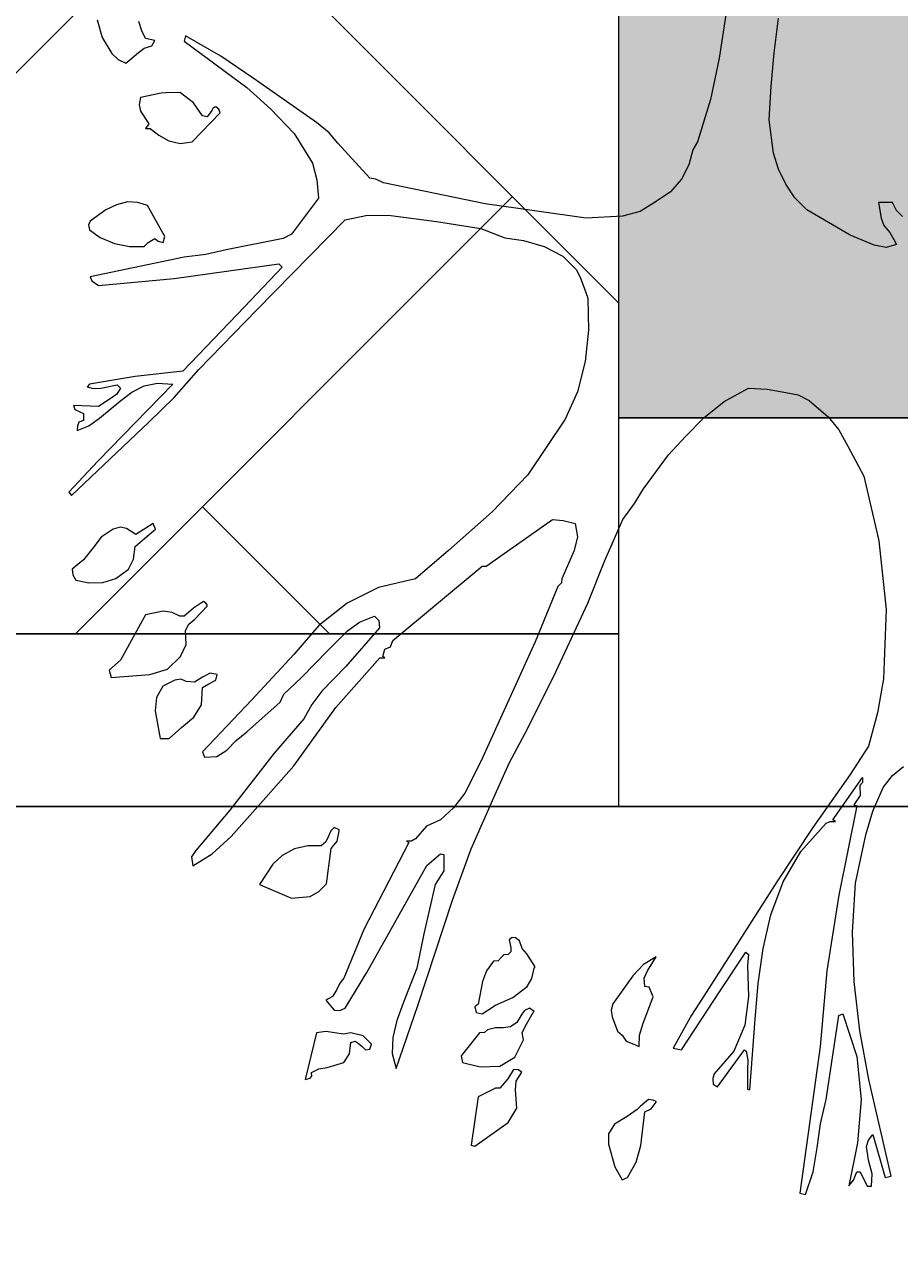
# Model space of a CAD drawing. Units: inches. Extents: x 84 to 1044, y -280 to 906.
# Tile 3 of 105: x 441 to 462, y -132 to -104. Entities that reach past the tile are written whole.
import ezdxf

# ---------------------------------------------------------------- set-up
doc = ezdxf.new("R2010")
doc.units = ezdxf.units.IN
for name, color, linetype, lineweight in [('A-ANNO-DIMS', 2, 'Continuous', 18), ('C-PROP', 7, 'Continuous', 25), ('L-HRDS', 32, 'Continuous', 18), ('L-PLNT', 114, 'Continuous', 15)]:
    doc.layers.add(name, color=color, linetype=linetype, lineweight=lineweight)
doc.layers.add('L-PLNT-PATT', color=9, linetype='Continuous', lineweight=9, true_color=0xafd9aa)
doc.layers.add('L-PRKG-PATT', color=35, linetype='Continuous', lineweight=9, true_color=0x947764)
doc.styles.get("Standard").update_dxf_attribs({"font": 'arial.ttf'})
doc.dimstyles.get("Standard").update_dxf_attribs({"dimtxt": 0.18, "dimasz": 0.18, "dimexe": 0.18, "dimexo": 0.0625, "dimgap": 0.09, "dimtad": 0, "dimtih": 1, "dimtoh": 1, "dimdec": 4, "dimzin": 0, "dimdsep": 46, "dimtxsty": 'Standard', "dimcen": 0.09, "dimadec": 0, "dimazin": 0, "dimtfac": 1, "dimtdec": 4, "dimtofl": 0, "dimtmove": 0, "dimatfit": 3, "dimfxl": 1, "dimtolj": 1, "dimtzin": 0, "dimarcsym": 0})

# ---------------------------------------------------------------- blocks, each defined once
blk = doc.blocks.new('A$C37E508DF')
for p, q in [((0.7911, 1.1436), (0.8027, 1.0677)), ((0.7512, 1.0728), (0.7469, 1.1054)), ((1.3455, 1.0934), (1.3485, 1.102)), ((1.3875, 1.1037), (1.3828, 1.087)), ((1.2713, 1.0694), (1.3044, 1.0887)), ((1.3044, 1.0887), (1.3057, 1.0835)), ((1.3421, 1.0861), (1.3455, 1.0934)), ((1.3057, 1.0835), (1.2469, 1.0402)), ((1.3335, 1.0844), (1.3421, 1.0861)), ((1.3361, 1.0793), (1.3335, 1.0844)), ((1.3434, 1.0771), (1.3361, 1.0793)), ((1.349, 1.0728), (1.3434, 1.0771)), ((1.3828, 1.087), (1.3738, 1.072)), ((0.7538, 1.0415), (0.7512, 1.0728)), ((0.8027, 1.0677), (0.8108, 1.0287)), ((1.2409, 1.0488), (1.2713, 1.0694)), ((1.3605, 1.063), (1.349, 1.0728)), ((1.3678, 1.0664), (1.3605, 1.063)), ((1.3738, 1.072), (1.3678, 1.0664)), ((1.1813, 1.0072), (1.2409, 1.0488)), ((0.7559, 1.0098), (0.7538, 1.0415)), ((1.2469, 1.0402), (1.2246, 1.0201)), ((1.2971, 1.0257), (1.3091, 1.0351)), ((1.3091, 1.0351), (1.3185, 1.0355)), ((1.3185, 1.0355), (1.3275, 1.0347)), ((1.3275, 1.0347), (1.3468, 1.0308)), ((0.8108, 1.0287), (0.8233, 0.9892)), ((1.2246, 1.0201), (1.2023, 0.9969)), ((1.2718, 1.0162), (1.2731, 1.0197)), ((1.2731, 1.0197), (1.2761, 1.0218)), ((1.2761, 1.0218), (1.2786, 1.0209)), ((1.2786, 1.0209), (1.2799, 1.0184)), ((1.2885, 1.0136), (1.2971, 1.0257)), ((1.3468, 1.0308), (1.3481, 1.0239)), ((1.3481, 1.0239), (1.3468, 1.018)), ((0.7516, 0.9785), (0.7559, 1.0098)), ((1.2984, 0.9892), (1.2718, 1.0162)), ((1.2799, 1.0184), (1.2842, 1.0124)), ((1.2842, 1.0124), (1.2885, 1.0136)), ((1.3468, 1.018), (1.3391, 1.0059)), ((1.1612, 0.9879), (1.1693, 0.9974)), ((1.1693, 0.9974), (1.1813, 1.0072)), ((1.2023, 0.9969), (1.1852, 0.9691)), ((1.3378, 1.0016), (1.3297, 0.9952)), ((1.3421, 1.0016), (1.3378, 1.0016)), ((1.3391, 1.0059), (1.3421, 1.0016)), ((0.8233, 0.9892), (0.8275, 0.9815)), ((1.1311, 0.9549), (1.1612, 0.9879)), ((1.3095, 0.9875), (1.2984, 0.9892)), ((1.3202, 0.9901), (1.3095, 0.9875)), ((1.3297, 0.9952), (1.3202, 0.9901)), ((0.7469, 0.9635), (0.7516, 0.9785)), ((0.8275, 0.9815), (0.8314, 0.9673)), ((0.7401, 0.9493), (0.7469, 0.9635)), ((0.8314, 0.9673), (0.8383, 0.954)), ((1.1852, 0.9691), (1.1809, 0.9532)), ((0.8383, 0.954), (0.8486, 0.942)), ((1.1183, 0.9506), (1.1256, 0.954)), ((1.1256, 0.954), (1.1311, 0.9549)), ((1.1809, 0.9532), (1.1796, 0.936)), ((0.7315, 0.9365), (0.7401, 0.9493)), ((0.8486, 0.942), (0.8619, 0.933)), ((1.0227, 0.9309), (1.1183, 0.9506)), ((0.6359, 0.9245), (0.6397, 0.9322)), ((0.6397, 0.9322), (0.653, 0.9322)), ((0.653, 0.9322), (0.6505, 0.9172)), ((0.7203, 0.9253), (0.7315, 0.9365)), ((0.8619, 0.933), (0.8769, 0.9236)), ((0.9279, 0.9172), (1.0227, 0.9309)), ((1.1796, 0.936), (1.2049, 0.9022)), ((1.3241, 0.9), (1.3404, 0.9292)), ((1.3404, 0.9292), (1.3494, 0.9322)), ((1.3494, 0.9322), (1.3592, 0.9326)), ((1.3592, 0.9326), (1.3695, 0.93)), ((1.3695, 0.93), (1.3794, 0.9253)), ((0.6303, 0.9189), (0.6359, 0.9245)), ((0.6505, 0.9172), (0.6479, 0.9103)), ((0.6796, 0.9013), (0.7203, 0.9253)), ((0.8769, 0.9236), (0.8936, 0.9193)), ((0.8936, 0.9193), (0.9279, 0.9172)), ((1.1114, 0.9198), (1.0685, 0.9142)), ((1.1333, 0.9202), (1.1114, 0.9198)), ((1.1543, 0.9159), (1.1333, 0.9202)), ((1.3794, 0.9253), (1.394, 0.9146)), ((0.6479, 0.9103), (0.6423, 0.9039)), ((1.0269, 0.9077), (1.0042, 0.8987)), ((1.0685, 0.9142), (1.0269, 0.9077)), ((1.2371, 0.8314), (1.1543, 0.9159)), ((1.3948, 0.9065), (1.3846, 0.8992)), ((1.394, 0.9146), (1.3957, 0.9112)), ((1.3957, 0.9112), (1.3948, 0.9065)), ((0.6384, 0.8974), (0.6359, 0.8927)), ((0.6423, 0.9039), (0.6384, 0.8974)), ((0.6569, 0.8919), (0.6796, 0.9013)), ((0.9866, 0.8962), (0.9673, 0.8906)), ((1.0042, 0.8987), (0.9866, 0.8962)), ((1.2049, 0.9022), (1.2126, 0.8983)), ((1.2126, 0.8983), (1.2662, 0.8876)), ((1.3254, 0.8944), (1.3241, 0.9)), ((1.3301, 0.8957), (1.3254, 0.8944)), ((1.3335, 0.8983), (1.3301, 0.8957)), ((1.3395, 0.8944), (1.3335, 0.8983)), ((1.3434, 0.8906), (1.3395, 0.8944)), ((1.3713, 0.8936), (1.3571, 0.8906)), ((1.3846, 0.8992), (1.3713, 0.8936)), ((0.6359, 0.8927), (0.6457, 0.8897)), ((0.6457, 0.8897), (0.6569, 0.8919)), ((0.9673, 0.8906), (0.9498, 0.8816)), ((1.2662, 0.8876), (1.2855, 0.8833)), ((1.2855, 0.8833), (1.3057, 0.8807)), ((1.3571, 0.8906), (1.3434, 0.8906)), ((0.9498, 0.8816), (0.9369, 0.8687)), ((1.2169, 0.8743), (1.2135, 0.8713)), ((1.2135, 0.8713), (1.2491, 0.834)), ((1.3151, 0.8606), (1.2169, 0.8743)), ((1.3057, 0.8807), (1.394, 0.8623)), ((0.933, 0.861), (0.9296, 0.852)), ((0.9369, 0.8687), (0.933, 0.861)), ((1.3863, 0.8541), (1.3151, 0.8606)), ((1.394, 0.8623), (1.3927, 0.8584)), ((0.9296, 0.852), (0.9262, 0.8421)), ((1.3927, 0.8584), (1.3863, 0.8541)), ((0.9262, 0.8421), (0.9257, 0.8121)), ((1.2919, 0.7752), (1.2371, 0.8314)), ((1.2491, 0.834), (1.3069, 0.7735)), ((0.9257, 0.8121), (0.9287, 0.7825)), ((0.9287, 0.7825), (0.936, 0.7542)), ((1.3151, 0.7487), (1.2919, 0.7752)), ((1.3069, 0.7735), (1.352, 0.7684)), ((1.352, 0.7684), (1.3948, 0.7615)), ((0.7577, 0.7568), (0.7401, 0.7534)), ((0.7752, 0.7577), (0.7577, 0.7568)), ((0.798, 0.7452), (0.7752, 0.7577)), ((1.3309, 0.7624), (1.3164, 0.7615)), ((1.3164, 0.7615), (1.3871, 0.6891)), ((1.3434, 0.7598), (1.3309, 0.7624)), ((1.355, 0.7538), (1.3434, 0.7598)), ((1.3687, 0.7607), (1.3657, 0.7577)), ((1.3657, 0.7577), (1.3691, 0.7521)), ((1.3841, 0.7577), (1.3687, 0.7607)), ((1.3914, 0.7572), (1.3841, 0.7577)), ((1.397, 0.759), (1.3914, 0.7572)), ((1.3948, 0.7615), (1.397, 0.759)), ((0.7182, 0.7461), (0.7002, 0.7307)), ((0.7285, 0.7512), (0.7182, 0.7461)), ((0.7401, 0.7534), (0.7285, 0.7512)), ((0.8173, 0.7298), (0.798, 0.7452)), ((0.936, 0.7542), (0.9476, 0.7285)), ((1.3391, 0.7255), (1.3151, 0.7487)), ((1.3653, 0.7461), (1.355, 0.7538)), ((1.3854, 0.7294), (1.3653, 0.7461)), ((1.3691, 0.7521), (1.3743, 0.7482)), ((1.3743, 0.7482), (1.3863, 0.7405)), ((1.3863, 0.7405), (1.4099, 0.7414)), ((1.4086, 0.7375), (1.4004, 0.7337)), ((1.4004, 0.7337), (1.4004, 0.7272)), ((1.4099, 0.7414), (1.4086, 0.7375)), ((0.7002, 0.7307), (0.6903, 0.7186)), ((0.8344, 0.7122), (0.8173, 0.7298)), ((0.9476, 0.7285), (0.9828, 0.6762)), ((1.4116, 0.6569), (1.3391, 0.7255)), ((1.3953, 0.7221), (1.3854, 0.7294)), ((1.4064, 0.7178), (1.3953, 0.7221)), ((1.4004, 0.7272), (1.4047, 0.7255)), ((1.4047, 0.7255), (1.406, 0.7221)), ((1.406, 0.7221), (1.4064, 0.7178)), ((0.6903, 0.7186), (0.6818, 0.7032)), ((0.8503, 0.6951), (0.8344, 0.7122)), ((0.6818, 0.7032), (0.6667, 0.6749)), ((0.8739, 0.6629), (0.8503, 0.6951)), ((1.3871, 0.6891), (1.4141, 0.6599)), ((0.9828, 0.6762), (1.0162, 0.6415)), ((0.6667, 0.6749), (0.6526, 0.614)), ((0.8824, 0.6492), (0.8739, 0.6629)), ((1.4141, 0.6599), (1.4116, 0.6569)), ((0.8932, 0.6342), (0.8824, 0.6492)), ((0.9103, 0.5956), (0.8932, 0.6342)), ((0.9382, 0.6303), (0.936, 0.6179)), ((0.9493, 0.6333), (0.9382, 0.6303)), ((0.9596, 0.6342), (0.9493, 0.6333)), ((1.0218, 0.5904), (0.9596, 0.6342)), ((1.0162, 0.6415), (1.0574, 0.605)), ((1.3327, 0.6252), (1.3348, 0.6303)), ((1.3348, 0.6303), (1.3511, 0.62)), ((1.343, 0.6162), (1.3327, 0.6252)), ((1.3511, 0.62), (1.3601, 0.6256)), ((1.3601, 0.6256), (1.3661, 0.6269)), ((1.3661, 0.6269), (1.3725, 0.6252)), ((1.3725, 0.6252), (1.3837, 0.6175)), ((0.6526, 0.614), (0.6457, 0.5497)), ((0.936, 0.6179), (0.939, 0.605)), ((1.352, 0.6089), (1.343, 0.6162)), ((1.3533, 0.5969), (1.352, 0.6089)), ((1.3837, 0.6175), (1.3918, 0.6072)), ((0.939, 0.605), (0.9506, 0.5784)), ((1.0574, 0.605), (1.0883, 0.5784)), ((1.358, 0.5874), (1.3533, 0.5969)), ((1.3918, 0.6072), (1.4004, 0.5964)), ((1.4004, 0.5964), (1.4111, 0.5874)), ((0.9262, 0.5557), (0.9103, 0.5956)), ((1.0256, 0.5904), (1.0218, 0.5904)), ((1.1097, 0.5205), (1.0256, 0.5904)), ((1.37, 0.5789), (1.358, 0.5874)), ((1.4111, 0.5874), (1.4103, 0.5823)), ((0.9506, 0.5784), (0.951, 0.5746)), ((0.951, 0.5746), (0.9545, 0.5711)), ((1.0883, 0.5784), (1.123, 0.5703)), ((1.3824, 0.575), (1.37, 0.5789)), ((1.3953, 0.5746), (1.3824, 0.575)), ((1.4077, 0.5771), (1.3953, 0.5746)), ((1.4103, 0.5823), (1.4077, 0.5771)), ((0.9545, 0.5711), (0.9759, 0.5193)), ((1.123, 0.5703), (1.1526, 0.5557)), ((0.9583, 0.4871), (0.9262, 0.5557)), ((1.1526, 0.5557), (1.1792, 0.5347)), ((1.2842, 0.554), (1.2855, 0.5557)), ((1.2842, 0.5527), (1.2842, 0.554)), ((1.2958, 0.5407), (1.2842, 0.5527)), ((1.2855, 0.5557), (1.2876, 0.557)), ((1.2876, 0.557), (1.2971, 0.551)), ((1.2971, 0.551), (1.3057, 0.5433)), ((0.6457, 0.5497), (0.6483, 0.4845)), ((1.1226, 0.5394), (1.1221, 0.5325)), ((1.1268, 0.5433), (1.1226, 0.5394)), ((1.141, 0.5377), (1.1268, 0.5433)), ((1.3014, 0.536), (1.2958, 0.5407)), ((1.3057, 0.5433), (1.3099, 0.5433)), ((1.3099, 0.5433), (1.3172, 0.5467)), ((1.3172, 0.5467), (1.3254, 0.548)), ((1.3254, 0.548), (1.3421, 0.5446)), ((1.3421, 0.5446), (1.3657, 0.5021)), ((1.1221, 0.5325), (1.1539, 0.4961)), ((1.1521, 0.5296), (1.141, 0.5377)), ((1.1706, 0.5111), (1.1521, 0.5296)), ((1.1792, 0.5347), (1.2027, 0.5072)), ((1.3044, 0.53), (1.3014, 0.536)), ((1.3039, 0.5167), (1.3044, 0.53)), ((0.9759, 0.5193), (1.0269, 0.4069)), ((1.1118, 0.5145), (1.1097, 0.5205)), ((1.3091, 0.5055), (1.3039, 0.5167)), ((1.117, 0.5124), (1.1118, 0.5145)), ((1.1191, 0.5055), (1.117, 0.5124)), ((1.117, 0.5042), (1.1191, 0.5055)), ((1.1217, 0.5042), (1.117, 0.5042)), ((1.1633, 0.4575), (1.1217, 0.5042)), ((1.1955, 0.4858), (1.1706, 0.5111)), ((1.2027, 0.5072), (1.2426, 0.4644)), ((1.3215, 0.4935), (1.3091, 0.5055)), ((1.1539, 0.4961), (1.1762, 0.4729)), ((1.3382, 0.4884), (1.3215, 0.4935)), ((1.3657, 0.5021), (1.3764, 0.4927)), ((1.3764, 0.4927), (1.3743, 0.4858)), ((0.6483, 0.4845), (0.6539, 0.4524)), ((0.9853, 0.4335), (0.9583, 0.4871)), ((1.207, 0.4747), (1.1955, 0.4858)), ((1.2748, 0.4884), (1.2812, 0.4897)), ((1.2761, 0.4832), (1.2748, 0.4884)), ((1.2825, 0.4798), (1.2761, 0.4832)), ((1.2812, 0.4897), (1.2885, 0.4862)), ((1.2885, 0.4862), (1.2962, 0.4815)), ((1.2962, 0.4815), (1.3039, 0.482)), ((1.3039, 0.482), (1.3087, 0.4841)), ((1.3087, 0.4841), (1.3147, 0.4832)), ((1.3147, 0.4832), (1.3258, 0.4777)), ((1.3743, 0.4858), (1.3382, 0.4884)), ((1.1762, 0.4729), (1.1856, 0.4605)), ((1.2122, 0.47), (1.207, 0.4747)), ((1.2156, 0.4627), (1.2122, 0.47)), ((1.2885, 0.4764), (1.2825, 0.4798)), ((1.2894, 0.4601), (1.2885, 0.4764)), ((1.3258, 0.4777), (1.3318, 0.4669)), ((1.1856, 0.4605), (1.1933, 0.4468)), ((1.2469, 0.4348), (1.2156, 0.4627)), ((1.2426, 0.4644), (1.2885, 0.4159)), ((1.2967, 0.4485), (1.2894, 0.4601)), ((1.3318, 0.4669), (1.3331, 0.4545)), ((0.6539, 0.4524), (0.6625, 0.4211)), ((1.2027, 0.4026), (1.1633, 0.4575)), ((1.1933, 0.4468), (1.2212, 0.4146)), ((1.3082, 0.4386), (1.2967, 0.4485)), ((1.3331, 0.4545), (1.3284, 0.4284)), ((1.3198, 0.4284), (1.3082, 0.4386)), ((1.0003, 0.4052), (0.9853, 0.4335)), ((1.2568, 0.4266), (1.2469, 0.4348)), ((1.2658, 0.4176), (1.2568, 0.4266)), ((1.3284, 0.4284), (1.3198, 0.4284)), ((0.6625, 0.4211), (0.6796, 0.3945)), ((1.2212, 0.4146), (1.2628, 0.361)), ((1.2752, 0.4116), (1.2658, 0.4176)), ((1.2885, 0.4159), (1.2868, 0.4108)), ((0.6397, 0.3936), (0.6295, 0.4022)), ((1.0145, 0.373), (1.0003, 0.4052)), ((1.0269, 0.4069), (1.0419, 0.3769)), ((1.2289, 0.373), (1.2027, 0.4026)), ((1.2868, 0.4108), (1.2752, 0.4116)), ((0.6487, 0.3825), (0.6397, 0.3936)), ((0.6959, 0.352), (0.668, 0.3919)), ((0.668, 0.3919), (0.668, 0.3872)), ((0.6796, 0.3945), (0.7148, 0.3447)), ((0.6582, 0.3602), (0.6487, 0.3825)), ((0.668, 0.3872), (0.6706, 0.3842)), ((0.6706, 0.3842), (0.6702, 0.3748)), ((0.6702, 0.3748), (0.6762, 0.3662)), ((1.0359, 0.3246), (1.0145, 0.373)), ((1.0419, 0.3769), (1.0527, 0.3632)), ((1.2615, 0.3362), (1.2289, 0.373)), ((0.665, 0.3379), (0.6582, 0.3602)), ((0.6762, 0.3662), (0.6732, 0.3653)), ((0.6732, 0.3653), (0.6903, 0.2813)), ((1.0527, 0.3632), (1.0647, 0.352)), ((1.2628, 0.361), (1.2949, 0.3233)), ((0.6933, 0.3503), (0.6959, 0.352)), ((0.6985, 0.3503), (0.6933, 0.3503)), ((0.7023, 0.349), (0.6985, 0.3503)), ((0.7259, 0.3224), (0.7023, 0.349)), ((0.7148, 0.3447), (0.7487, 0.2937)), ((1.0647, 0.352), (1.078, 0.346)), ((1.078, 0.346), (1.0883, 0.334)), ((1.1599, 0.3426), (1.1646, 0.3447)), ((1.1646, 0.3447), (1.168, 0.3417)), ((0.6745, 0.2924), (0.665, 0.3379)), ((1.0883, 0.334), (1.0921, 0.3319)), ((1.1599, 0.3413), (1.1599, 0.3426)), ((1.162, 0.3319), (1.1599, 0.3413)), ((1.168, 0.3417), (1.1702, 0.3366)), ((1.1702, 0.3366), (1.1727, 0.3314)), ((1.2795, 0.3199), (1.2615, 0.3362)), ((0.7427, 0.2937), (0.7259, 0.3224)), ((1.0535, 0.2766), (1.0359, 0.3246)), ((1.0921, 0.3319), (1.0968, 0.3319)), ((1.0968, 0.3319), (1.0947, 0.3306)), ((1.0947, 0.3306), (1.1367, 0.2491)), ((1.1676, 0.325), (1.162, 0.3319)), ((1.1719, 0.292), (1.1676, 0.325)), ((1.1727, 0.3314), (1.177, 0.3276)), ((1.177, 0.3276), (1.1895, 0.3276)), ((1.1895, 0.3276), (1.2019, 0.3246)), ((1.2019, 0.3246), (1.2135, 0.3186)), ((1.2949, 0.3233), (1.2988, 0.3173)), ((1.0647, 0.3199), (1.0617, 0.3194)), ((1.0617, 0.3194), (1.0617, 0.304)), ((1.0711, 0.3147), (1.0647, 0.3199)), ((1.0775, 0.3092), (1.0711, 0.3147)), ((1.2135, 0.3186), (1.2225, 0.3104)), ((1.2225, 0.3104), (1.2349, 0.2911)), ((1.2975, 0.3087), (1.2795, 0.3199)), ((1.2988, 0.3173), (1.2975, 0.3087)), ((1.0617, 0.304), (1.0698, 0.2911)), ((1.1341, 0.2084), (1.0775, 0.3092)), ((0.6775, 0.2465), (0.6745, 0.2924)), ((0.7542, 0.2628), (0.7427, 0.2937)), ((0.7487, 0.2937), (0.8151, 0.1899)), ((1.0698, 0.2911), (1.0805, 0.2448)), ((1.1792, 0.2847), (1.1719, 0.292)), ((1.2349, 0.2911), (1.2049, 0.2783)), ((0.6903, 0.2813), (0.7015, 0.2101)), ((1.0861, 0.1775), (1.0535, 0.2766)), ((1.1873, 0.28), (1.1792, 0.2847)), ((1.2049, 0.2783), (1.1873, 0.28)), ((0.7615, 0.2311), (0.7542, 0.2628)), ((0.6758, 0.2002), (0.6775, 0.2465)), ((0.9905, 0.2384), (0.9943, 0.241)), ((0.9943, 0.241), (0.9973, 0.2414)), ((0.9973, 0.2414), (1.0003, 0.2393)), ((1.0805, 0.2448), (1.087, 0.2127)), ((1.1367, 0.2491), (1.1556, 0.2032)), ((0.7662, 0.1981), (0.7615, 0.2311)), ((0.9836, 0.226), (0.9879, 0.2311)), ((0.9879, 0.2311), (0.9905, 0.2384)), ((1.0003, 0.2393), (0.9986, 0.232)), ((0.9986, 0.232), (0.9986, 0.2281)), ((0.7778, 0.2277), (0.7752, 0.2255)), ((0.7752, 0.2255), (0.7761, 0.2152)), ((0.8018, 0.1912), (0.7778, 0.2277)), ((0.8619, 0.2234), (0.8739, 0.2161)), ((0.87, 0.2101), (0.8619, 0.2234)), ((0.9759, 0.214), (0.9836, 0.226)), ((0.9986, 0.2281), (1.0012, 0.2255)), ((1.0012, 0.2255), (1.0051, 0.2251)), ((1.0051, 0.2251), (1.0076, 0.2225)), ((1.0076, 0.2225), (1.0106, 0.2195)), ((1.0106, 0.2195), (1.0149, 0.2191)), ((1.0149, 0.2191), (1.0214, 0.2101)), ((0.7015, 0.2101), (0.7079, 0.1389)), ((0.7761, 0.2152), (0.7752, 0.1861)), ((0.8734, 0.2032), (0.87, 0.2101)), ((0.8739, 0.2161), (0.8841, 0.2054)), ((0.9768, 0.2127), (0.9759, 0.214)), ((0.9789, 0.2028), (0.9768, 0.2127)), ((1.0214, 0.2101), (1.0252, 0.2002)), ((1.087, 0.2127), (1.0998, 0.1797)), ((1.1543, 0.1749), (1.1341, 0.2084)), ((0.6706, 0.1539), (0.6758, 0.2002)), ((0.7688, 0.1646), (0.7662, 0.1981)), ((0.8687, 0.1947), (0.8726, 0.1955)), ((0.8726, 0.1955), (0.8734, 0.2032)), ((0.8841, 0.2054), (0.9026, 0.1792)), ((0.9832, 0.1955), (0.9789, 0.2028)), ((0.9969, 0.1852), (0.9832, 0.1955)), ((1.0252, 0.2002), (1.0295, 0.1788)), ((1.1556, 0.2032), (1.1594, 0.1985)), ((1.1594, 0.1985), (1.1624, 0.1921)), ((0.7752, 0.1861), (0.7787, 0.1591)), ((0.8383, 0.1359), (0.8018, 0.1912)), ((0.8151, 0.1899), (0.8288, 0.1685)), ((0.8649, 0.1857), (0.8687, 0.1947)), ((0.8743, 0.1608), (0.8649, 0.1857)), ((1.0132, 0.1779), (0.9969, 0.1852)), ((1.1624, 0.1921), (1.1663, 0.1861)), ((1.1663, 0.1861), (1.1727, 0.1827)), ((0.9026, 0.1792), (0.9043, 0.1732)), ((0.9043, 0.1732), (0.9035, 0.1668)), ((0.9768, 0.1719), (0.9811, 0.1749)), ((0.9776, 0.1711), (0.9768, 0.1719)), ((0.9811, 0.1749), (0.9858, 0.1728)), ((0.9858, 0.1728), (0.9884, 0.1694)), ((1.0256, 0.1698), (1.0132, 0.1779)), ((1.0295, 0.1788), (1.0325, 0.1762)), ((1.0325, 0.1762), (1.0312, 0.1711)), ((1.1063, 0.1183), (1.0861, 0.1775)), ((1.0998, 0.1797), (1.1058, 0.1634)), ((1.1594, 0.1728), (1.1543, 0.1749)), ((1.1646, 0.1732), (1.1594, 0.1728)), ((1.1727, 0.1827), (1.1646, 0.1732)), ((0.6865, 0.1698), (0.6732, 0.1295)), ((0.6903, 0.1681), (0.6865, 0.1698)), ((0.7023, 0.0892), (0.6903, 0.1681)), ((0.774, 0.0982), (0.7688, 0.1646)), ((0.8288, 0.1685), (0.846, 0.1376)), ((0.8777, 0.1496), (0.8743, 0.1608)), ((0.9035, 0.1668), (0.8983, 0.1535)), ((0.9853, 0.1578), (0.9776, 0.1711)), ((0.9884, 0.1694), (0.9931, 0.1616)), ((0.9931, 0.1616), (0.9991, 0.1574)), ((1.0312, 0.1711), (1.0256, 0.1698)), ((1.1058, 0.1634), (1.1097, 0.1475)), ((0.662, 0.108), (0.6706, 0.1539)), ((0.7787, 0.1591), (0.789, 0.1346)), ((0.8781, 0.1389), (0.8777, 0.1496)), ((0.894, 0.1496), (0.8902, 0.1441)), ((0.8983, 0.1535), (0.894, 0.1496)), ((0.9879, 0.1518), (0.9853, 0.1578)), ((0.9866, 0.1453), (0.9879, 0.1518)), ((0.9991, 0.1574), (1.0059, 0.1565)), ((1.0059, 0.1565), (1.0132, 0.1565)), ((1.0132, 0.1565), (1.0205, 0.1548)), ((1.0205, 0.1548), (1.0235, 0.1522)), ((1.0235, 0.1522), (1.0282, 0.1518)), ((1.0282, 0.1518), (1.0454, 0.1303)), ((1.1298, 0.1411), (1.1376, 0.1492)), ((1.1376, 0.1492), (1.1491, 0.1518)), ((1.1491, 0.1518), (1.1564, 0.1505)), ((1.1564, 0.1505), (1.1642, 0.1518)), ((1.1642, 0.1518), (1.1727, 0.1531)), ((1.1727, 0.1531), (1.1813, 0.1518)), ((1.1813, 0.1518), (1.192, 0.108)), ((0.7079, 0.1389), (0.7268, 0.0013)), ((0.846, 0.1376), (0.8383, 0.1359)), ((0.8846, 0.1419), (0.8781, 0.1389)), ((0.8902, 0.1441), (0.8846, 0.1419)), ((0.9948, 0.1291), (0.9866, 0.1453)), ((1.1097, 0.1475), (1.1101, 0.1325)), ((1.1311, 0.1364), (1.1298, 0.1411)), ((1.1384, 0.1389), (1.1354, 0.1359)), ((1.1423, 0.1423), (1.1384, 0.1389)), ((1.1449, 0.1441), (1.1423, 0.1423)), ((1.1491, 0.1428), (1.1449, 0.1441)), ((1.1504, 0.132), (1.1491, 0.1428)), ((0.6732, 0.1295), (0.6693, 0.0892)), ((0.7774, 0.1346), (0.7757, 0.1261)), ((0.7757, 0.1261), (0.7761, 0.117)), ((0.7791, 0.1359), (0.7774, 0.1346)), ((0.8044, 0.1012), (0.7791, 0.1359)), ((0.789, 0.1346), (0.8074, 0.1132)), ((1.0089, 0.1205), (0.9948, 0.1291)), ((1.0454, 0.1303), (1.0441, 0.1239)), ((1.1101, 0.1325), (1.1063, 0.1183)), ((1.1354, 0.1359), (1.1311, 0.1364)), ((1.1556, 0.1239), (1.1504, 0.132)), ((0.7761, 0.117), (0.7761, 0.099)), ((0.9884, 0.1149), (0.9918, 0.117)), ((0.9935, 0.1063), (0.9884, 0.1149)), ((0.9918, 0.117), (0.9961, 0.1175)), ((0.9961, 0.1175), (1.0016, 0.1085)), ((1.0274, 0.12), (1.0089, 0.1205)), ((1.0441, 0.1239), (1.0274, 0.12)), ((1.1714, 0.1192), (1.1556, 0.1239)), ((1.1792, 0.1179), (1.1714, 0.1192)), ((1.186, 0.1145), (1.1792, 0.1179)), ((0.641, 0.0172), (0.662, 0.108)), ((0.8083, 0.1037), (0.8044, 0.1012)), ((0.8074, 0.1132), (0.8087, 0.1089)), ((0.8087, 0.1089), (0.8083, 0.1037)), ((0.9943, 0.0982), (0.9935, 0.1063)), ((1.0016, 0.1085), (1.0089, 0.0999)), ((1.1856, 0.111), (1.186, 0.1145)), ((1.1873, 0.1093), (1.1856, 0.111)), ((1.192, 0.108), (1.1873, 0.1093)), ((0.7761, 0.099), (0.774, 0.0982)), ((0.9931, 0.081), (0.9943, 0.0982)), ((1.0089, 0.0999), (1.0132, 0.0999)), ((1.0132, 0.0999), (1.0295, 0.0917)), ((1.0295, 0.0917), (1.0359, 0.0463)), ((0.6693, 0.0892), (0.6728, 0.0484)), ((0.7075, 0.0665), (0.7023, 0.0892)), ((0.8619, 0.0875), (0.8649, 0.0887)), ((0.8619, 0.0866), (0.8619, 0.0875)), ((0.8666, 0.0806), (0.8619, 0.0866)), ((0.8649, 0.0887), (0.8691, 0.0892)), ((0.8726, 0.0776), (0.8666, 0.0806)), ((0.8691, 0.0892), (0.8769, 0.0827)), ((0.8769, 0.0827), (0.8799, 0.0797)), ((1.0012, 0.0677), (0.9931, 0.081)), ((0.8764, 0.0459), (0.8726, 0.0776)), ((0.8799, 0.0797), (0.8893, 0.0733)), ((0.8893, 0.0733), (0.9013, 0.066)), ((0.7105, 0.0437), (0.7075, 0.0665)), ((0.9013, 0.066), (0.9069, 0.057)), ((1.0325, 0.0454), (1.0012, 0.0677)), ((0.6582, 0.0562), (0.6466, 0.0159)), ((0.6625, 0.051), (0.6582, 0.0562)), ((0.6642, 0.045), (0.6625, 0.051)), ((0.6728, 0.0484), (0.6809, 0.0082)), ((0.8807, 0.0304), (0.8764, 0.0459)), ((0.9069, 0.0471), (0.9009, 0.0261)), ((0.9069, 0.057), (0.9069, 0.0471)), ((1.0359, 0.0463), (1.0325, 0.0454)), ((0.6625, 0.0321), (0.6642, 0.045)), ((0.7144, 0.0214), (0.7105, 0.0437)), ((0.659, 0.0193), (0.6625, 0.0321)), ((0.8889, 0.0159), (0.8807, 0.0304)), ((0.9009, 0.0261), (0.894, 0.0137)), ((0.6466, 0.0159), (0.641, 0.0172)), ((0.6595, 0.0077), (0.659, 0.0193)), ((0.6702, 0.0214), (0.6637, 0.0077)), ((0.6732, 0.0214), (0.6702, 0.0214)), ((0.6766, 0.0133), (0.6732, 0.0214)), ((0.6809, 0.0082), (0.6766, 0.0133)), ((0.7216, 0), (0.7144, 0.0214)), ((0.894, 0.0137), (0.8889, 0.0159)), ((0.6637, 0.0077), (0.6595, 0.0077)), ((0.7268, 0.0013), (0.7216, 0))]:
    blk.add_line(p, q)
blk = doc.blocks.new('*D60')
at = {"layer": 'A-ANNO-DIMS', "color": 0, "lineweight": -2, "transparency": 16777216}
for p, q in [((134.179, -121.942), (134.179, -180.64)), ((992.074, -121.942), (992.074, -180.64)), ((134.359, -180.46), (562.733, -180.46)), ((991.894, -180.46), (563.521, -180.46))]:
    blk.add_line(p, q, dxfattribs=at)
at = {"layer": 'A-ANNO-DIMS', "color": 0, "transparency": 16777216}
for points in [[(134.359, -180.43), (134.359, -180.49), (134.179, -180.46)], [(991.894, -180.43), (991.894, -180.49), (992.074, -180.46)]]:
    blk.add_solid(points, dxfattribs=at)
at = {"layer": 'Defpoints', "color": 0, "transparency": 16777216}
for p in [(134.179, -121.88), (992.074, -121.88), (992.074, -180.46)]:
    blk.add_point(p, dxfattribs=at)
at = {"layer": 'A-ANNO-DIMS', "color": 0, "transparency": 16777216, "insert": (563.127, -180.46), "char_height": 0.18, "attachment_point": 5}
blk.add_mtext('\\A1;857.9', dxfattribs=at)

msp = doc.modelspace()

# ---------------------------------------------------------------- hatches: boundary and pattern name
at = {"layer": 'L-PLNT-PATT', "transparency": 33554597}
h = msp.add_hatch(color=256, dxfattribs=at)
h.dxf.hatch_style = 1
h.paths.add_polyline_path([(504.574, -40.88), (455.074, -40.88), (455.074, -112.88), (504.574, -112.88)])
at = {"layer": 'L-PRKG-PATT', "transparency": 33554567}
h = msp.add_hatch(dxfattribs=at)
h.set_pattern_fill('AR-HBONE', color=256, scale=0.1)
h.paths.add_polyline_path([(455.074, 31.12), (455.074, 91.12), (455.074, 151.12), (413.127, 151.12), (341.127, 151.12), (290.179, 151.12), (227.179, 151.12), (227.179, 127.12), (143.179, 127.12), (143.179, -112.88), (143.179, -117.88), (455.074, -117.88)])

# ---------------------------------------------------------------- linework, layer by layer
at = {"layer": 'C-PROP'}
for p, q in [((143.179, -117.88), (455.074, -117.88)), ((143.179, -121.88), (455.074, -121.88))]:
    msp.add_line(p, q, dxfattribs=at)
for points in [[(504.574, -112.88), (455.074, -112.88)], [(504.574, -121.88), (455.074, -121.88)]]:
    msp.add_lwpolyline(points, dxfattribs=at)
at = {"layer": 'L-HRDS'}
msp.add_line((455.074, 31.12), (455.074, -121.88), dxfattribs=at)

# ---------------------------------------------------------------- block references
at = {"layer": 'L-PLNT', "xscale": -24.64361536662419, "yscale": 24.64361536662419, "zscale": 24.64361536662419}
msp.add_blockref('A$C37E508DF', (477.187, -130.86), dxfattribs=at)

# ---------------------------------------------------------------- dimensions: what is measured, and where the dimension line sits
at = {"layer": 'A-ANNO-DIMS'}
dim = msp.add_linear_dim(base=(992.074, -180.46), p1=(134.179, -121.88), p2=(992.074, -121.88), dimstyle='Standard', override={"dimdec": 1, "dimlfac": 1, "dimrnd": 0, "dimzin": 0, "dimdsep": 46, "dimlunit": 2}, dxfattribs=at)
dim.commit()
dim.dimension.update_dxf_attribs({"geometry": '*D60', "text_midpoint": (563.127, -180.46)})

doc.saveas('drawing.dxf')
